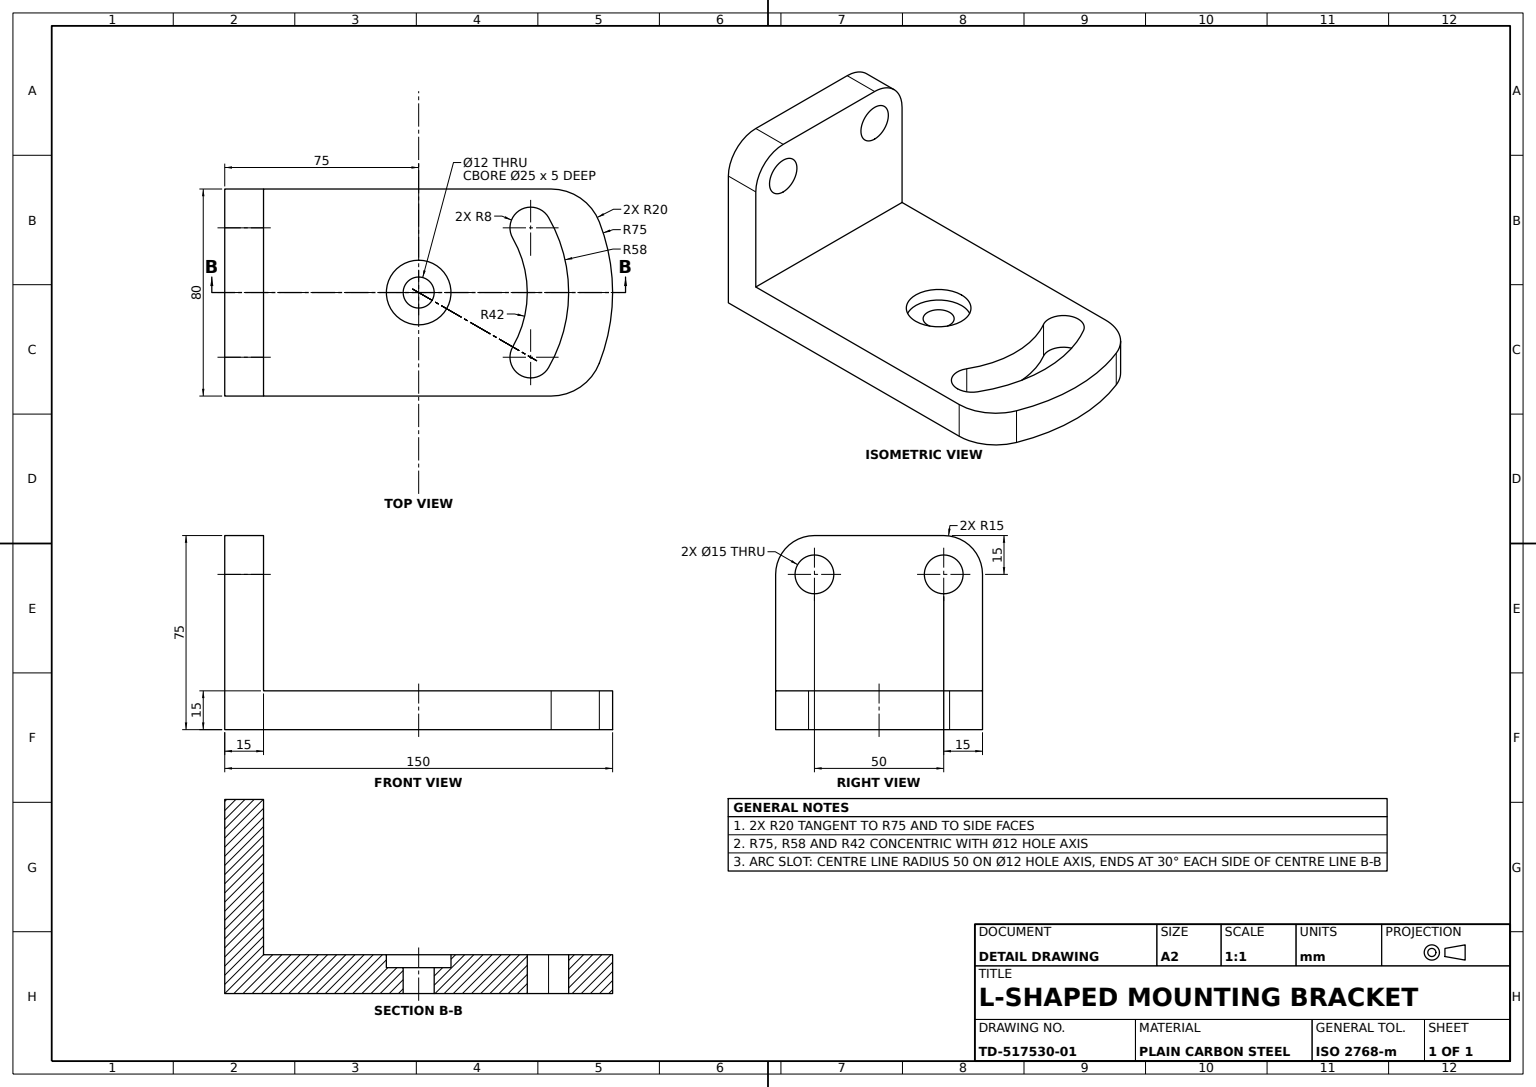
from build123d import *
from OCP.BRepFilletAPI import BRepFilletAPI_MakeFillet

# Parameters (mm, degrees)
L_BRACKET_BODY_DEPTH             = 40
ARC_SLOT_R50_30DEG_REACH         = 168.433
CORNER_ROUNDS_R1                 = 20
CORNER_ROUNDS_R2                 = 15
COUNTERBORED_HOLE_12_D           = 12
COUNTERBORED_HOLE_12_DEPTH       = 100
COUNTERBORED_HOLE_12_CBORE_D     = 25
COUNTERBORED_HOLE_12_CBORE_DEPTH = 5
UPRIGHT_HOLES_2X_REACH           = 161.531
UPRIGHT_HOLES_SKETCH_R           = 7.5


with BuildPart() as part:
    # L Profile Sketch → L Bracket Body (new, symmetric)
    with BuildSketch(Plane.XY):
        Polygon((0, 0), (0, 75), (15, 75), (15, 15), (150, 15), (150, 0), align=None)
    extrude(amount=L_BRACKET_BODY_DEPTH, both=True)

    # Arc Slot Sketch → Arc Slot R50 30deg (cut, up to next)
    with BuildSketch(Plane(origin=(0, 15, 0), x_dir=(1, 0, 0), z_dir=(0, 1, 0)), mode=Mode.PRIVATE) as arc_slot_r50_30deg_sk1:
        with BuildLine():
            Line((138.442887702, -40), (150, -40))
            Line((150, -40), (150, 0))
            ThreePointArc((150, 0), (147.052815967, -20.818062138), (138.442887702, -40))
        make_face()
    arc_slot_r50_30deg_tool1 = extrude(arc_slot_r50_30deg_sk1.sketch, amount=-ARC_SLOT_R50_30DEG_REACH, mode=Mode.PRIVATE) & part.part
    # Arc Slot Sketch → Arc Slot R50 30deg (cut, up to next)
    with BuildSketch(Plane(origin=(0, 15, 0), x_dir=(1, 0, 0), z_dir=(0, 1, 0)), mode=Mode.PRIVATE) as arc_slot_r50_30deg_sk2:
        with BuildLine():
            ThreePointArc((138.442887702, 40), (147.052815967, 20.818062138), (150, 0))
            Line((150, 0), (150, 40))
            Line((150, 40), (138.442887702, 40))
        make_face()
    arc_slot_r50_30deg_tool2 = extrude(arc_slot_r50_30deg_sk2.sketch, amount=-ARC_SLOT_R50_30DEG_REACH, mode=Mode.PRIVATE) & part.part
    # Arc Slot Sketch → Arc Slot R50 30deg (cut, up to next)
    with BuildSketch(Plane(origin=(0, 15, 0), x_dir=(1, 0, 0), z_dir=(0, 1, 0)), mode=Mode.PRIVATE) as arc_slot_r50_30deg_sk3:
        with BuildLine():
            ThreePointArc((125.229473419, -29), (133, 0), (125.229473419, 29))
            ThreePointArc((125.229473419, 29), (114.301270189, 31.92820323), (111.373066959, 21))
            ThreePointArc((111.373066959, 21), (117, 0), (111.373066959, -21))
            ThreePointArc((111.373066959, -21), (114.301270189, -31.92820323), (125.229473419, -29))
        make_face()
    arc_slot_r50_30deg_tool3 = extrude(arc_slot_r50_30deg_sk3.sketch, amount=-ARC_SLOT_R50_30DEG_REACH, mode=Mode.PRIVATE) & part.part
    add(arc_slot_r50_30deg_tool1.solids().sort_by_distance((146.584015, 15, 30.160634))[0], mode=Mode.SUBTRACT)
    add(arc_slot_r50_30deg_tool2.solids().sort_by_distance((146.584015, 15, -30.160634))[0], mode=Mode.SUBTRACT)
    add(arc_slot_r50_30deg_tool3.solids().sort_by_distance((121.886119, 15, 0))[0], mode=Mode.SUBTRACT)

    # Corner Rounds: one fillet with a radius per group of edges: ONE call of the kernel's fillet builder (fillet() takes one radius for all edges)
    corner_rounds_edges_1 = [part.edges().sort_by_distance(p)[0] for p in [
        (138.442887702, 7.5, 40),
        (138.442887702, 7.5, -40),
    ]]
    corner_rounds_edges_2 = [part.edges().sort_by_distance(p)[0] for p in [
        (7.5, 75, 40),
        (7.5, 75, -40),
    ]]
    corner_rounds = BRepFilletAPI_MakeFillet(part.part.solid().wrapped)
    for e in corner_rounds_edges_1:
        corner_rounds.Add(CORNER_ROUNDS_R1, e.wrapped)
    for e in corner_rounds_edges_2:
        corner_rounds.Add(CORNER_ROUNDS_R2, e.wrapped)
    add(Compound.cast(corner_rounds.Shape()), mode=Mode.REPLACE)

    # Counterbored Hole _12
    with Locations(Plane(origin=(0, 15, 0), x_dir=(1, 0, 0), z_dir=(0, 1, 0))):
        with Locations((75, 0)):
            CounterBoreHole(COUNTERBORED_HOLE_12_D / 2, COUNTERBORED_HOLE_12_CBORE_D / 2, COUNTERBORED_HOLE_12_CBORE_DEPTH, depth=COUNTERBORED_HOLE_12_DEPTH)

    # Upright Holes Sketch → Upright Holes 2x (cut, up to next)
    with BuildSketch(Plane(origin=(15, 0, 0), x_dir=(0, 0, -1), z_dir=(1, 0, 0)), mode=Mode.PRIVATE) as upright_holes_2x_sk1:
        with Locations(Location((-25, 60, 0), (0, 0, 90))):
            Circle(UPRIGHT_HOLES_SKETCH_R)
    upright_holes_2x_tool1 = extrude(upright_holes_2x_sk1.sketch, amount=-UPRIGHT_HOLES_2X_REACH, mode=Mode.PRIVATE) & part.part
    # Upright Holes Sketch → Upright Holes 2x (cut, up to next)
    with BuildSketch(Plane(origin=(15, 0, 0), x_dir=(0, 0, -1), z_dir=(1, 0, 0)), mode=Mode.PRIVATE) as upright_holes_2x_sk2:
        with Locations(Location((25, 60, 0), (0, 0, 90))):
            Circle(UPRIGHT_HOLES_SKETCH_R)
    upright_holes_2x_tool2 = extrude(upright_holes_2x_sk2.sketch, amount=-UPRIGHT_HOLES_2X_REACH, mode=Mode.PRIVATE) & part.part
    add(upright_holes_2x_tool1.solids().sort_by_distance((15, 60, 25))[0], mode=Mode.SUBTRACT)
    add(upright_holes_2x_tool2.solids().sort_by_distance((15, 60, -25))[0], mode=Mode.SUBTRACT)


solid = part.part
